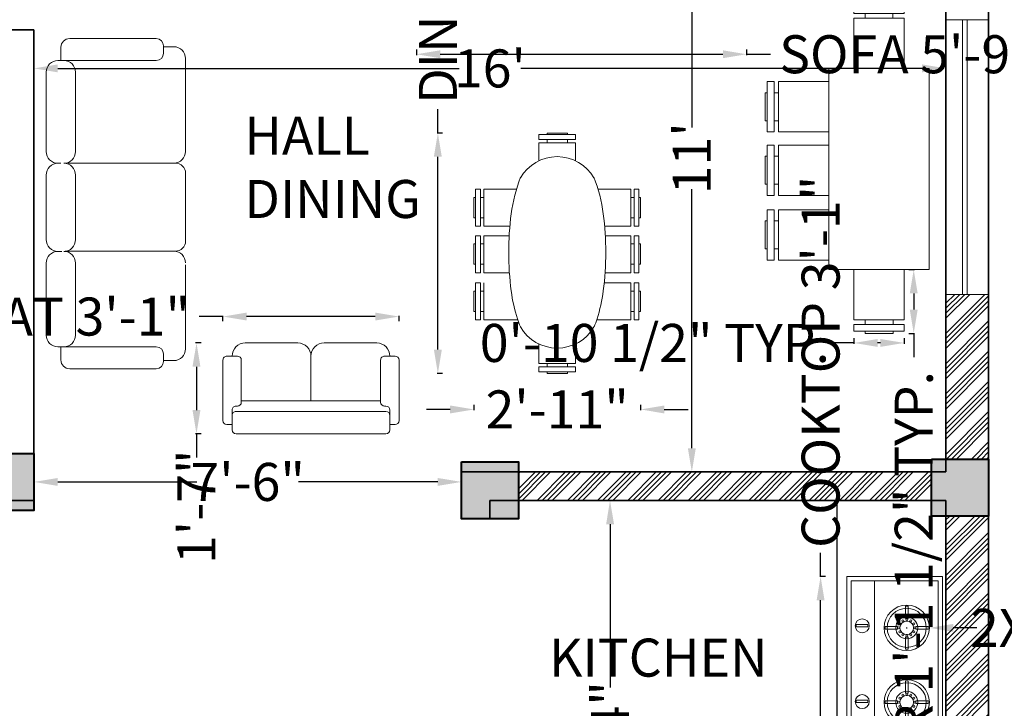
# Model space of a CAD drawing. Units: inches. Extents: x -52 to 493, y -432 to 100.
# Tile 3 of 5: x 163 to 370, y -300 to -155. Entities that reach past the tile are written whole.
import ezdxf

# ---------------------------------------------------------------- set-up
doc = ezdxf.new("R2010")
doc.units = ezdxf.units.IN
doc.header["$MEASUREMENT"] = 0
for name, color, linetype, lineweight in [('A-ANNO-DIMS', 2, 'Continuous', 18), ('A-AREA-IDEN', 7, 'Continuous', 25), ('A-COLS', 7, 'Continuous', 40), ('A-EQPM', 8, 'Continuous', 18), ('A-FLOR-CASE', 8, 'Continuous', 25), ('A-FURN', 8, 'Continuous', 18), ('A-GLAZ', 4, 'Continuous', 18), ('A-WALL', 7, 'Continuous', 35), ('A-WALL-PATT', 8, 'Continuous', 13)]:
    doc.layers.add(name, color=color, linetype=linetype, lineweight=lineweight)
doc.styles.get("Standard").update_dxf_attribs({"font": 'arial.ttf'})
doc.dimstyles.get("Standard").update_dxf_attribs({"dimtxt": 8, "dimasz": 5, "dimexe": 0.18, "dimexo": 0.0625, "dimgap": 0.09, "dimtad": 0, "dimdec": 0, "dimzin": 0, "dimdsep": 46, "dimlunit": 3, "dimtxsty": 'Standard', "dimcen": 0.09, "dimadec": 0, "dimazin": 0, "dimtfac": 1, "dimtdec": 0, "dimtofl": 0, "dimtmove": 0, "dimatfit": 3, "dimfxl": 1, "dimfxlon": 1, "dimtolj": 1, "dimtzin": 0, "dimarcsym": 0})

# ---------------------------------------------------------------- blocks, each defined once
blk = doc.blocks.new('A$C39D66038')
for p, q in [((0.656, 2.02), (0.656, 1.96)), ((1.106, 2.02), (0.656, 2.02)), ((1.106, 1.96), (0.656, 1.96)), ((1.006, 2.04), (0.756, 2.04)), ((0.756, 2.04), (0.756, 2.02)), ((0.756, 1.96), (0.756, 1.92)), ((1.006, 2.02), (1.006, 2.04)), ((1.006, 1.92), (1.006, 1.96)), ((1.106, 1.96), (1.106, 2.02)), ((1.684, 2.02), (1.232, 2.02)), ((1.232, 2.02), (1.232, 1.96)), ((1.684, 1.96), (1.232, 1.96)), ((1.584, 2.04), (1.334, 2.04)), ((1.334, 2.04), (1.334, 2.02)), ((1.334, 1.96), (1.334, 1.92)), ((1.584, 2.02), (1.584, 2.04)), ((1.584, 1.92), (1.584, 1.96)), ((1.684, 1.96), (1.684, 2.02)), ((2.252, 2.02), (1.802, 2.02)), ((1.802, 2.02), (1.802, 1.96)), ((2.252, 1.96), (1.802, 1.96)), ((2.152, 2.04), (1.902, 2.04)), ((1.902, 2.04), (1.902, 2.02)), ((1.902, 1.96), (1.902, 1.92)), ((2.152, 2.02), (2.152, 2.04)), ((2.152, 1.92), (2.152, 1.96)), ((2.252, 1.96), (2.252, 2.02)), ((0.656, 1.92), (0.656, 1.503)), ((1.106, 1.92), (0.656, 1.92)), ((1.232, 1.92), (1.232, 1.606)), ((1.684, 1.92), (1.232, 1.92)), ((1.684, 1.609), (1.684, 1.92)), ((2.252, 1.92), (1.802, 1.92)), ((1.802, 1.92), (1.802, 1.6)), ((2.252, 1.52), (2.252, 1.92)), ((0.02, 1.245), (0.02, 0.795)), ((0.08, 1.245), (0.02, 1.245)), ((0.08, 1.245), (0.08, 0.795)), ((0.12, 1.245), (0.12, 0.795)), ((0.36, 1.245), (0.12, 1.245)), ((2.82, 1.245), (2.6, 1.245)), ((2.82, 0.795), (2.82, 1.245)), ((2.86, 0.795), (2.86, 1.245)), ((2.92, 1.245), (2.86, 1.245)), ((2.92, 0.795), (2.92, 1.245)), ((0, 1.145), (0, 0.895)), ((0.02, 1.145), (0, 1.145)), ((0.12, 1.145), (0.08, 1.145)), ((2.86, 1.145), (2.82, 1.145)), ((2.94, 1.145), (2.92, 1.145)), ((2.94, 0.895), (2.94, 1.145)), ((0, 0.895), (0.02, 0.895)), ((0.08, 0.895), (0.12, 0.895)), ((2.82, 0.895), (2.86, 0.895)), ((2.92, 0.895), (2.94, 0.895)), ((0.02, 0.795), (0.08, 0.795)), ((0.12, 0.795), (0.36, 0.795)), ((2.6, 0.795), (2.82, 0.795)), ((2.86, 0.795), (2.92, 0.795)), ((0.656, 0.537), (0.656, 0.12)), ((2.252, 0.12), (2.252, 0.52)), ((1.106, 0.12), (1.106, 0.445)), ((1.232, 0.434), (1.232, 0.12)), ((1.684, 0.12), (1.684, 0.431)), ((1.802, 0.44), (1.802, 0.12)), ((0.656, 0.12), (1.106, 0.12)), ((0.656, 0.08), (1.106, 0.08)), ((0.656, 0.08), (0.656, 0.02)), ((0.656, 0.02), (1.106, 0.02)), ((0.756, 0.12), (0.756, 0.08)), ((0.756, 0.02), (0.756, 0)), ((1.006, 0.08), (1.006, 0.12)), ((1.006, 0), (1.006, 0.02)), ((1.106, 0.02), (1.106, 0.08)), ((1.232, 0.12), (1.684, 0.12)), ((1.232, 0.08), (1.684, 0.08)), ((1.232, 0.08), (1.232, 0.02)), ((1.232, 0.02), (1.684, 0.02)), ((1.334, 0.12), (1.334, 0.08)), ((1.334, 0.02), (1.334, 0)), ((1.584, 0.08), (1.584, 0.12)), ((1.584, 0), (1.584, 0.02)), ((1.684, 0.02), (1.684, 0.08)), ((1.802, 0.12), (2.252, 0.12)), ((1.802, 0.08), (2.252, 0.08)), ((1.802, 0.08), (1.802, 0.02)), ((1.802, 0.02), (2.252, 0.02)), ((1.902, 0.12), (1.902, 0.08)), ((1.902, 0.02), (1.902, 0)), ((2.152, 0.08), (2.152, 0.12)), ((2.152, 0), (2.152, 0.02)), ((2.252, 0.02), (2.252, 0.08)), ((0.756, 0), (1.006, 0)), ((1.334, 0), (1.584, 0)), ((1.902, 0), (2.152, 0))]:
    blk.add_line(p, q)
for centre, radius, start, end in [((1.267, -0.378), 1.978, 97.5169, 107.6698), ((1.48, -1.99), 3.604, 90, 97.5169), ((1.48, -1.99), 3.604, 82.4831, 90), ((1.693, -0.378), 1.978, 69.0857, 82.4831), ((0.827, 1.02), 0.518, 119.7736, 240.2264), ((0.946, 0.63), 0.921, 107.6698, 114.1273), ((2.133, 1.02), 0.518, 299.7736, 60.2264), ((0.946, 1.41), 0.921, 245.8727, 252.3302), ((1.267, 2.418), 1.978, 252.3302, 262.4831), ((1.693, 2.418), 1.978, 277.5169, 290.9143), ((1.48, 4.03), 3.604, 262.4831, 270), ((1.48, 4.03), 3.604, 270, 277.5169)]:
    blk.add_arc(centre, radius, start, end)
blk = doc.blocks.new('A$C0876780F')
for p, q in [((0.72, 0.95), (0.23, 0.95)), ((1.32, 0.95), (0.88, 0.95)), ((1.48, 0.95), (2.02, 0.95)), ((0.15, 0.85), (0.06, 0.85)), ((0.15, 0.87), (0.15, 0.8444)), ((0.15, 0.87), (0.15, 0.85)), ((0.15, 0.21), (0.15, 0.85)), ((0.8, 0.85), (0.8, 0.87)), ((0.8, 0.87), (0.8, 0.85)), ((0.8, 0.87), (0.8, 0.8444)), ((0.8011, 0.8204), (0.8011, 0.08)), ((1.4, 0.85), (1.4, 0.87)), ((1.4, 0.85), (1.4, 0.87)), ((2.1, 0.87), (2.1, 0.85)), ((2.1, 0.87), (2.1, 0.8444)), ((2.1, 0.21), (2.1, 0.85)), ((2.1, 0.85), (2.19, 0.85)), ((0, 0.79), (0, 0.21)), ((0.72, 0.75), (0.23, 0.75)), ((1.32, 0.75), (0.88, 0.75)), ((1.4014, 0.08), (1.4014, 0.803)), ((1.48, 0.75), (2.02, 0.75)), ((2.25, 0.79), (2.25, 0.21)), ((0, 0.21), (0, 0.2)), ((0.15, 0.2), (0.15, 0.25)), ((2.1, 0.2), (2.1, 0.25)), ((2.25, 0.21), (2.25, 0.2)), ((0.05, 0.15), (0.1, 0.15)), ((0.056, 0.15), (0.056, 0.08)), ((2.2, 0.15), (2.15, 0.15)), ((2.194, 0.15), (2.194, 0.08)), ((0.8011, 0.07), (0.8011, 0.08)), ((1.4014, 0.07), (1.4014, 0.08)), ((0.136, 0), (0.7093, 0)), ((0.8711, 0), (1.3314, 0)), ((2.114, 0), (1.48, 0))]:
    blk.add_line(p, q)
for centre, radius, start, end in [((0.23, 0.87), 0.08, 90, 180), ((0.72, 0.87), 0.08, 0, 90), ((0.88, 0.87), 0.08, 90, 180), ((1.32, 0.87), 0.08, 0, 90), ((1.48, 0.87), 0.08, 90, 180), ((2.02, 0.87), 0.08, 0, 90), ((0.06, 0.79), 0.06, 90, 180), ((0.23, 0.83), 0.08, 180, 270), ((0.23, 0.83), 0.08, 180, 270), ((0.72, 0.83), 0.08, 270, 0), ((0.88, 0.83), 0.08, 180, 270), ((0.88, 0.83), 0.08, 180, 270), ((1.32, 0.83), 0.08, 270, 0), ((1.48, 0.83), 0.08, 180, 270), ((2.02, 0.83), 0.08, 270, 0), ((2.02, 0.83), 0.08, 270, 0), ((2.19, 0.79), 0.06, 0, 90), ((0.09, 0.21), 0.06, 350.53768, 0), ((2.16, 0.21), 0.06, 180, 189.46232), ((0.05, 0.2), 0.05, 180, 270), ((0.1, 0.2), 0.05, 270, 0), ((2.15, 0.2), 0.05, 180, 270), ((2.2, 0.2), 0.05, 270, 0), ((0.136, 0.08), 0.08, 180, 270), ((0.7211, 0.08), 0.08, 270, 0), ((0.8711, 0.07), 0.07, 180, 270), ((1.3314, 0.07), 0.07, 270, 0), ((1.4814, 0.08), 0.08, 180, 270), ((2.114, 0.08), 0.08, 270, 0)]:
    blk.add_arc(centre, radius, start, end)
blk = doc.blocks.new('A$C02A636C4')
for p, q in [((1.2026, 0.6692), (0.097, 0.6692)), ((0.0679, 0.6013), (0.0291, 0.6013)), ((0.0679, 0.6401), (0.0679, 0.6013)), ((0.0679, 0.5334), (0.0679, 0.6013)), ((1.2317, 0.6401), (1.2317, 0.6013)), ((1.2317, 0.6013), (1.2705, 0.6013)), ((1.2317, 0.5334), (1.2317, 0.6013)), ((0, 0.5722), (0, 0.1261)), ((0.0679, 0.4946), (0.0679, 0.5431)), ((1.2317, 0.4946), (1.2317, 0.5431)), ((1.2996, 0.5722), (1.2996, 0.1261)), ((1.2026, 0.5043), (0.097, 0.5043)), ((0.1067, 0.4655), (0.097, 0.4655)), ((0.1358, 0.1261), (0.1358, 0.4364)), ((1.1638, 0.1261), (1.1638, 0.4364)), ((1.1929, 0.4655), (1.2026, 0.4655)), ((1.1638, 0.4267), (0.1358, 0.4267)), ((0.6498, 0.097), (0.6498, 0.4267)), ((0.0291, 0.097), (0.1067, 0.097)), ((1.2705, 0.097), (1.1929, 0.097)), ((0.1649, 0), (0.5528, 0)), ((0.7468, 0), (1.1347, 0))]:
    blk.add_line(p, q)
for centre, radius, start, end in [((0.097, 0.6401), 0.0291, 90, 180), ((1.2026, 0.6401), 0.0291, 0, 90), ((0.0291, 0.5722), 0.0291, 90, 180), ((1.2705, 0.5722), 0.0291, 0, 90), ((0.097, 0.5334), 0.0291, 180, 270), ((1.2026, 0.5334), 0.0291, 270, 0), ((0.097, 0.4946), 0.0291, 180, 270), ((0.1067, 0.4364), 0.0291, 0, 90), ((1.1929, 0.4364), 0.0291, 90, 180), ((1.2026, 0.4946), 0.0291, 270, 0), ((0.0291, 0.1261), 0.0291, 180, 270), ((0.1649, 0.097), 0.097, 180, 270), ((0.1067, 0.1261), 0.0291, 270, 0), ((0.5528, 0.097), 0.097, 270, 0), ((0.7468, 0.097), 0.097, 180, 270), ((1.1347, 0.097), 0.097, 270, 0), ((1.1929, 0.1261), 0.0291, 180, 270), ((1.2705, 0.1261), 0.0291, 270, 0)]:
    blk.add_arc(centre, radius, start, end)
blk = doc.blocks.new('A$C06E242FC')
for p, q in [((0, 455.6), (0.5, 456.1)), ((0, 455.6), (0, 0.5)), ((838.9, 456.1), (0.5, 456.1)), ((20, 435.6), (20.5, 436.1)), ((20, 435.6), (20, 20.5)), ((818.9, 436.1), (20.5, 436.1)), ((819.4, 435.6), (818.9, 436.1)), ((819.4, 20.5), (819.4, 435.6)), ((838.9, 456.1), (839.4, 455.6)), ((839.4, 0.5), (839.4, 455.6)), ((237.3, 411.5), (237.3, 356.2)), ((248.9, 411.5), (237.3, 411.5)), ((248.9, 356.2), (248.9, 411.5)), ((599.3, 411.5), (610.9, 411.5)), ((599.3, 411.5), (599.3, 356.2)), ((610.9, 356.2), (610.9, 411.5)), ((237.3, 356.2), (248.9, 356.2)), ((599.3, 356.2), (610.9, 356.2)), ((20, 324.4), (819.4, 324.4)), ((232.7, 272.7), (232.7, 214)), ((244.9, 272.7), (232.7, 272.7)), ((244.9, 214), (244.9, 272.7)), ((588.1, 272.7), (588.1, 214)), ((600.3, 272.7), (588.1, 272.7)), ((600.3, 214), (600.3, 272.7)), ((232.7, 214), (244.9, 214)), ((588.1, 214), (600.3, 214)), ((136.3, 176), (136.3, 163.8)), ((194.9, 176), (136.3, 176)), ((136.3, 163.8), (194.9, 163.8)), ((194.9, 163.8), (194.9, 176)), ((282.9, 176.3), (282.9, 164.1)), ((341.6, 176.3), (282.9, 176.3)), ((282.9, 164.1), (341.6, 164.1)), ((341.6, 164.1), (341.6, 176.3)), ((550.3, 176), (491.7, 176)), ((491.7, 176), (491.7, 163.8)), ((491.7, 163.8), (550.3, 163.8)), ((550.3, 163.8), (550.3, 176)), ((638.3, 176.3), (638.3, 164.1)), ((697, 176.3), (638.3, 176.3)), ((638.3, 164.1), (697, 164.1)), ((697, 164.1), (697, 176.3)), ((245.2, 126.1), (233, 126.1)), ((233, 126.1), (233, 67.4)), ((245.2, 67.4), (245.2, 126.1)), ((600.6, 126.1), (588.3, 126.1)), ((588.3, 126.1), (588.3, 67.4)), ((600.6, 67.4), (600.6, 126.1)), ((233, 67.4), (245.2, 67.4)), ((588.3, 67.4), (600.6, 67.4)), ((0, 0.5), (0.5, 0)), ((20, 20.5), (20.5, 20)), ((20.5, 20), (818.9, 20)), ((818.9, 20), (819.4, 20.5)), ((838.9, 0), (839.4, 0.5)), ((0.5, 0), (838.9, 0))]:
    blk.add_line(p, q)
for centre, radius in [((242, 382.9), 33.3), ((604.1, 382.9), 33.3), ((238.9, 170.1), 108.3), ((238.9, 170.1), 93.3), ((594.3, 170.1), 108.3), ((594.3, 170.1), 93.3), ((238.9, 170.1), 52.6), ((205.3, 189.5), 4.84), ((238.9, 170.1), 32.6), ((219.5, 203.7), 4.84), ((238.9, 208.9), 4.84), ((258.4, 203.7), 4.84), ((272.6, 189.5), 4.84), ((594.3, 170.1), 52.6), ((560.7, 189.5), 4.84), ((594.3, 170.1), 32.6), ((574.9, 203.7), 4.84), ((594.3, 208.9), 4.84), ((613.7, 203.7), 4.84), ((628, 189.5), 4.84), ((200.1, 170.1), 4.84), ((205.3, 150.6), 4.84), ((219.5, 136.4), 4.84), ((258.4, 136.4), 4.84), ((272.6, 150.6), 4.84), ((277.8, 170.1), 4.84), ((555.5, 170.1), 4.84), ((560.7, 150.6), 4.84), ((574.9, 136.4), 4.84), ((613.7, 136.4), 4.84), ((628, 150.6), 4.84), ((633.2, 170.1), 4.84), ((238.9, 131.2), 4.84), ((594.3, 131.2), 4.84)]:
    blk.add_circle(centre, radius)
blk = doc.blocks.new('*D19')
at = {"layer": 'A-ANNO-DIMS', "color": 0, "lineweight": -2, "transparency": 16777216}
for p, q in [((285.94, -256.62), (287.12, -256.62)), ((286.94, -261.62), (286.94, -295.94)), ((286.94, -351.72), (286.94, -317.4)), ((285.94, -356.72), (287.12, -356.72))]:
    blk.add_line(p, q, dxfattribs=at)
at = {"layer": 'A-ANNO-DIMS', "color": 0, "transparency": 16777216}
for points in [[(286.11, -261.62), (287.78, -261.62), (286.94, -256.62)], [(286.11, -351.72), (287.78, -351.72), (286.94, -356.72)]]:
    blk.add_solid(points, dxfattribs=at)
at = {"layer": 'Defpoints', "color": 0, "transparency": 16777216}
for p in [(283.02, -256.62), (280.41, -356.72), (286.94, -356.72)]:
    blk.add_point(p, dxfattribs=at)
at = {"layer": 'A-ANNO-DIMS', "color": 0, "transparency": 16777216, "insert": (286.94, -306.67), "char_height": 8, "attachment_point": 5, "rotation": 90}
blk.add_mtext('\\A1;8\'-4"', dxfattribs=at)
blk = doc.blocks.new('*D24')
at = {"layer": 'A-ANNO-DIMS', "color": 0, "lineweight": -2, "transparency": 16777216}
for p, q in [((165.65, -252.71), (165.65, -252.53)), ((170.65, -252.71), (199.96, -252.71)), ((250.65, -252.71), (221.34, -252.71)), ((255.65, -252.71), (255.65, -252.53))]:
    blk.add_line(p, q, dxfattribs=at)
at = {"layer": 'A-ANNO-DIMS', "color": 0, "transparency": 16777216}
for points in [[(170.65, -251.88), (170.65, -253.54), (165.65, -252.71)], [(250.65, -251.88), (250.65, -253.54), (255.65, -252.71)]]:
    blk.add_solid(points, dxfattribs=at)
at = {"layer": 'Defpoints', "color": 0, "transparency": 16777216}
for p in [(165.65, -252.71), (255.65, -252.71), (255.65, -252.71)]:
    blk.add_point(p, dxfattribs=at)
at = {"layer": 'A-ANNO-DIMS', "color": 0, "transparency": 16777216, "insert": (210.65, -252.71), "char_height": 8, "attachment_point": 5}
blk.add_mtext('\\A1;7\'-6"', dxfattribs=at)
blk = doc.blocks.new('*D25')
at = {"layer": 'A-ANNO-DIMS', "color": 0, "lineweight": -2, "transparency": 16777216}
for p, q in [((165.65, -164.71), (165.65, -165.89)), ((170.65, -165.71), (255.15, -165.71)), ((352.65, -165.71), (268.15, -165.71)), ((357.65, -164.71), (357.65, -165.89))]:
    blk.add_line(p, q, dxfattribs=at)
at = {"layer": 'A-ANNO-DIMS', "color": 0, "transparency": 16777216}
for points in [[(170.65, -164.87), (170.65, -166.54), (165.65, -165.71)], [(352.65, -164.87), (352.65, -166.54), (357.65, -165.71)]]:
    blk.add_solid(points, dxfattribs=at)
at = {"layer": 'Defpoints', "color": 0, "transparency": 16777216}
for p in [(357.65, -155.46), (165.65, -160.73), (357.65, -165.71)]:
    blk.add_point(p, dxfattribs=at)
at = {"layer": 'A-ANNO-DIMS', "color": 0, "transparency": 16777216, "insert": (261.65, -165.71), "char_height": 8, "attachment_point": 5}
blk.add_mtext("\\A1;16'", dxfattribs=at)
blk = doc.blocks.new('*D26')
at = {"layer": 'A-ANNO-DIMS', "color": 0, "lineweight": -2, "transparency": 16777216}
for p, q in [((305.16, -118.62), (303.98, -118.62)), ((304.16, -123.62), (304.16, -178.11)), ((304.16, -245.62), (304.16, -191.12)), ((305.16, -250.62), (303.98, -250.62))]:
    blk.add_line(p, q, dxfattribs=at)
at = {"layer": 'A-ANNO-DIMS', "color": 0, "transparency": 16777216}
for points in [[(303.33, -123.62), (305, -123.62), (304.16, -118.62)], [(303.33, -245.62), (305, -245.62), (304.16, -250.62)]]:
    blk.add_solid(points, dxfattribs=at)
at = {"layer": 'Defpoints', "color": 0, "transparency": 16777216}
for p in [(304.16, -118.62), (307.2, -118.62), (312.14, -250.62)]:
    blk.add_point(p, dxfattribs=at)
at = {"layer": 'A-ANNO-DIMS', "color": 0, "transparency": 16777216, "insert": (304.16, -184.62), "char_height": 8, "attachment_point": 5, "rotation": 90}
blk.add_mtext("\\A1;11'", dxfattribs=at)
blk = doc.blocks.new('COL-12X12')
h = blk.add_hatch(color=256)
h.dxf.hatch_style = 1
h.paths.add_polyline_path([(12, 12), (0, 12), (0, 0), (12, 0)])
blk.add_lwpolyline([(0, 12), (12, 12), (12, 0), (0, 0)], close=True)
blk = doc.blocks.new('WIN-SIDE-58')
for p, q in [((0, 57.79), (9, 57.79)), ((3.5, 0), (3.5, 57.79)), ((4.5, 0), (4.5, 57.79)), ((0, 0), (9, 0))]:
    blk.add_line(p, q)
blk = doc.blocks.new('CHAIR-DINING')
for p, q in [((10.59, 12.94), (0, 12.94)), ((0, 12.94), (0, 11.53)), ((8.23, 13.41), (2.35, 13.41)), ((2.35, 13.41), (2.35, 12.94)), ((8.23, 12.94), (8.23, 13.41)), ((10.59, 11.53), (10.59, 12.94)), ((10.59, 11.53), (0, 11.53)), ((10.59, 10.59), (0, 10.59)), ((0, 10.59), (0, 0)), ((2.35, 11.53), (2.35, 10.59)), ((8.23, 10.59), (8.23, 11.53)), ((10.59, 0), (10.59, 10.59)), ((0, 0), (10.59, 0))]:
    blk.add_line(p, q)
blk = doc.blocks.new('*D44')
at = {"layer": 'A-ANNO-DIMS', "color": 0, "lineweight": -2, "transparency": 16777216}
for p, q in [((349.88, -208.05), (351.06, -208.05)), ((350.88, -213.05), (350.88, -216.46)), ((349.88, -221.46), (351.06, -221.46)), ((350.88, -221.46), (350.88, -226.46))]:
    blk.add_line(p, q, dxfattribs=at)
at = {"layer": 'A-ANNO-DIMS', "color": 0, "transparency": 16777216}
for points in [[(350.04, -213.05), (351.71, -213.05), (350.88, -208.05)], [(350.04, -216.46), (351.71, -216.46), (350.88, -221.46)]]:
    blk.add_solid(points, dxfattribs=at)
at = {"layer": 'Defpoints', "color": 0, "transparency": 16777216}
for p in [(348.87, -208.05), (348.87, -221.46), (350.88, -221.46)]:
    blk.add_point(p, dxfattribs=at)
at = {"layer": 'A-ANNO-DIMS', "color": 0, "transparency": 16777216, "insert": (350.88, -300.1), "char_height": 8, "attachment_point": 5, "rotation": 90}
blk.add_mtext('\\A1;DINING CHAIR 1\'-1 1/2" TYP.', dxfattribs=at)
blk = doc.blocks.new('*D45')
at = {"layer": 'A-ANNO-DIMS', "color": 0, "lineweight": -2, "transparency": 16777216}
for p, q in [((338.28, -223.47), (333.28, -223.47)), ((338.28, -222.47), (338.28, -223.65)), ((343.87, -223.47), (343.28, -223.47)), ((348.87, -222.47), (348.87, -223.65))]:
    blk.add_line(p, q, dxfattribs=at)
at = {"layer": 'A-ANNO-DIMS', "color": 0, "transparency": 16777216}
for points in [[(343.28, -222.64), (343.28, -224.3), (338.28, -223.47)], [(343.87, -222.64), (343.87, -224.3), (348.87, -223.47)]]:
    blk.add_solid(points, dxfattribs=at)
at = {"layer": 'Defpoints', "color": 0, "transparency": 16777216}
for p in [(338.28, -221.46), (348.87, -221.46), (338.28, -223.47)]:
    blk.add_point(p, dxfattribs=at)
at = {"layer": 'A-ANNO-DIMS', "color": 0, "transparency": 16777216, "insert": (296.38, -223.47), "char_height": 8, "attachment_point": 5}
blk.add_mtext('\\A1;0\'-10 1/2" TYP.', dxfattribs=at)
blk = doc.blocks.new('*D46')
at = {"layer": 'A-ANNO-DIMS', "color": 0, "lineweight": -2, "transparency": 16777216}
for p, q in [((246.2, -161.73), (246.2, -162.91)), ((251.2, -162.73), (310.69, -162.73)), ((315.69, -161.73), (315.69, -162.91)), ((315.69, -162.73), (320.69, -162.73))]:
    blk.add_line(p, q, dxfattribs=at)
at = {"layer": 'A-ANNO-DIMS', "color": 0, "transparency": 16777216}
for points in [[(251.2, -161.9), (251.2, -163.56), (246.2, -162.73)], [(310.69, -161.9), (310.69, -163.56), (315.69, -162.73)]]:
    blk.add_solid(points, dxfattribs=at)
at = {"layer": 'Defpoints', "color": 0, "transparency": 16777216}
for p in [(246.2, -152.31), (315.69, -152.31), (315.69, -162.73)]:
    blk.add_point(p, dxfattribs=at)
at = {"layer": 'A-ANNO-DIMS', "color": 0, "transparency": 16777216, "insert": (371.23, -162.73), "char_height": 8, "attachment_point": 5}
blk.add_mtext('\\A1;SOFA 5\'-9 1/2" TYP.', dxfattribs=at)
blk = doc.blocks.new('*D48')
at = {"layer": 'A-ANNO-DIMS', "color": 0, "lineweight": -2, "transparency": 16777216}
for p, q in [((250.69, -179.3), (250.69, -174.3)), ((251.69, -179.3), (250.51, -179.3)), ((250.69, -224.88), (250.69, -184.3)), ((251.69, -229.88), (250.51, -229.88))]:
    blk.add_line(p, q, dxfattribs=at)
at = {"layer": 'A-ANNO-DIMS', "color": 0, "transparency": 16777216}
for points in [[(249.85, -184.3), (251.52, -184.3), (250.69, -179.3)], [(249.85, -224.88), (251.52, -224.88), (250.69, -229.88)]]:
    blk.add_solid(points, dxfattribs=at)
at = {"layer": 'Defpoints', "color": 0, "transparency": 16777216}
for p in [(250.69, -179.3), (258.27, -179.3), (258.27, -229.88)]:
    blk.add_point(p, dxfattribs=at)
at = {"layer": 'A-ANNO-DIMS', "color": 0, "transparency": 16777216, "insert": (250.69, -120.92), "char_height": 8, "attachment_point": 5, "rotation": 90}
blk.add_mtext('\\A1;DINING SET 4\'-2 1/2"', dxfattribs=at)
blk = doc.blocks.new('*D49')
at = {"layer": 'A-ANNO-DIMS', "color": 0, "lineweight": -2, "transparency": 16777216}
for p, q in [((253.27, -237.46), (248.27, -237.46)), ((258.27, -236.46), (258.27, -237.64)), ((293.37, -236.46), (293.37, -237.64)), ((298.37, -237.46), (303.37, -237.46))]:
    blk.add_line(p, q, dxfattribs=at)
at = {"layer": 'A-ANNO-DIMS', "color": 0, "transparency": 16777216}
for points in [[(253.27, -236.63), (253.27, -238.3), (258.27, -237.46)], [(298.37, -236.63), (298.37, -238.3), (293.37, -237.46)]]:
    blk.add_solid(points, dxfattribs=at)
at = {"layer": 'Defpoints', "color": 0, "transparency": 16777216}
for p in [(258.27, -229.88), (293.37, -229.88), (258.27, -237.46)]:
    blk.add_point(p, dxfattribs=at)
at = {"layer": 'A-ANNO-DIMS', "color": 0, "transparency": 16777216, "insert": (275.82, -237.46), "char_height": 8, "attachment_point": 5}
blk.add_mtext('\\A1;2\'-11"', dxfattribs=at)
blk = doc.blocks.new('*D50')
at = {"layer": 'A-ANNO-DIMS', "color": 0, "lineweight": -2, "transparency": 16777216}
for p, q in [((205.43, -217.92), (200.43, -217.92)), ((205.43, -218.92), (205.43, -217.74)), ((237.52, -217.92), (210.43, -217.92)), ((242.52, -218.92), (242.52, -217.74))]:
    blk.add_line(p, q, dxfattribs=at)
at = {"layer": 'A-ANNO-DIMS', "color": 0, "transparency": 16777216}
for points in [[(210.43, -217.09), (210.43, -218.75), (205.43, -217.92)], [(237.52, -217.09), (237.52, -218.75), (242.52, -217.92)]]:
    blk.add_solid(points, dxfattribs=at)
at = {"layer": 'Defpoints', "color": 0, "transparency": 16777216}
for p in [(205.43, -217.92), (205.43, -223.48), (242.52, -223.48)]:
    blk.add_point(p, dxfattribs=at)
at = {"layer": 'A-ANNO-DIMS', "color": 0, "transparency": 16777216, "insert": (158.83, -217.92), "char_height": 8, "attachment_point": 5}
blk.add_mtext('\\A1;LOVESEAT 3\'-1"', dxfattribs=at)
blk = doc.blocks.new('*D51')
at = {"layer": 'A-ANNO-DIMS', "color": 0, "lineweight": -2, "transparency": 16777216}
for p, q in [((200.87, -223.48), (199.69, -223.48)), ((199.87, -228.48), (199.87, -237.58)), ((200.87, -242.58), (199.69, -242.58)), ((199.87, -242.58), (199.87, -247.58))]:
    blk.add_line(p, q, dxfattribs=at)
at = {"layer": 'A-ANNO-DIMS', "color": 0, "transparency": 16777216}
for points in [[(199.03, -228.48), (200.7, -228.48), (199.87, -223.48)], [(199.03, -237.58), (200.7, -237.58), (199.87, -242.58)]]:
    blk.add_solid(points, dxfattribs=at)
at = {"layer": 'Defpoints', "color": 0, "transparency": 16777216}
for p in [(205.43, -223.48), (199.87, -242.58), (205.43, -242.58)]:
    blk.add_point(p, dxfattribs=at)
at = {"layer": 'A-ANNO-DIMS', "color": 0, "transparency": 16777216, "insert": (199.87, -257.93), "char_height": 8, "attachment_point": 5, "rotation": 90}
blk.add_mtext('\\A1;1\'-7"', dxfattribs=at)
blk = doc.blocks.new('*D54')
at = {"layer": 'A-ANNO-DIMS', "color": 0, "lineweight": -2, "transparency": 16777216}
for p, q in [((331.27, -272.61), (331.27, -267.61)), ((332.27, -272.61), (331.09, -272.61)), ((331.27, -304.59), (331.27, -277.61)), ((332.27, -309.59), (331.09, -309.59))]:
    blk.add_line(p, q, dxfattribs=at)
at = {"layer": 'A-ANNO-DIMS', "color": 0, "transparency": 16777216}
for points in [[(330.43, -277.61), (332.1, -277.61), (331.27, -272.61)], [(330.43, -304.59), (332.1, -304.59), (331.27, -309.59)]]:
    blk.add_solid(points, dxfattribs=at)
at = {"layer": 'Defpoints', "color": 0, "transparency": 16777216}
for p in [(331.27, -272.61), (336.81, -272.61), (336.81, -309.59)]:
    blk.add_point(p, dxfattribs=at)
at = {"layer": 'A-ANNO-DIMS', "color": 0, "transparency": 16777216, "insert": (331.27, -227.44), "char_height": 8, "attachment_point": 5, "rotation": 90}
blk.add_mtext('\\A1;COOKTOP 3\'-1"', dxfattribs=at)
blk = doc.blocks.new('*D62')
at = {"layer": 'A-ANNO-DIMS', "color": 0, "lineweight": -2, "transparency": 16777216}
for p, q in [((390.3, -213.25), (390.3, -208.25)), ((389.3, -213.25), (390.48, -213.25)), ((390.3, -242.89), (390.3, -218.25)), ((389.3, -247.89), (390.48, -247.89))]:
    blk.add_line(p, q, dxfattribs=at)
at = {"layer": 'A-ANNO-DIMS', "color": 0, "transparency": 16777216}
for points in [[(389.46, -218.25), (391.13, -218.25), (390.3, -213.25)], [(389.46, -242.89), (391.13, -242.89), (390.3, -247.89)]]:
    blk.add_solid(points, dxfattribs=at)
at = {"layer": 'Defpoints', "color": 0, "transparency": 16777216}
for p in [(366.65, -213.25), (390.3, -213.25), (366.65, -247.89)]:
    blk.add_point(p, dxfattribs=at)
at = {"layer": 'A-ANNO-DIMS', "color": 0, "transparency": 16777216, "insert": (390.3, -185.03), "char_height": 8, "attachment_point": 5, "rotation": 90}
blk.add_mtext('\\A1;2\'-10 1/2"', dxfattribs=at)
blk = doc.blocks.new('*D73')
at = {"layer": 'A-ANNO-DIMS', "color": 0, "lineweight": -2, "transparency": 16777216}
for p, q in [((389.3, -260.49), (390.48, -260.49)), ((390.3, -265.49), (390.3, -269.69)), ((390.3, -295.34), (390.3, -291.13)), ((389.3, -300.34), (390.48, -300.34))]:
    blk.add_line(p, q, dxfattribs=at)
at = {"layer": 'A-ANNO-DIMS', "color": 0, "transparency": 16777216}
for points in [[(389.46, -265.49), (391.13, -265.49), (390.3, -260.49)], [(389.46, -295.34), (391.13, -295.34), (390.3, -300.34)]]:
    blk.add_solid(points, dxfattribs=at)
at = {"layer": 'Defpoints', "color": 0, "transparency": 16777216}
for p in [(261.65, -260.49), (261.65, -300.34), (390.3, -300.34)]:
    blk.add_point(p, dxfattribs=at)
at = {"layer": 'A-ANNO-DIMS', "color": 0, "transparency": 16777216, "insert": (390.3, -280.41), "char_height": 8, "attachment_point": 5, "rotation": 90}
blk.add_mtext('\\A1;3\'-4"', dxfattribs=at)
blk = doc.blocks.new('*D74')
at = {"layer": 'A-ANNO-DIMS', "color": 0, "lineweight": -2, "transparency": 16777216}
for p, q in [((334.72, 87.29), (334.72, 88.47)), ((339.72, 88.29), (352.65, 88.29)), ((357.65, 87.29), (357.65, 88.47)), ((357.65, 88.29), (362.65, 88.29))]:
    blk.add_line(p, q, dxfattribs=at)
at = {"layer": 'A-ANNO-DIMS', "color": 0, "transparency": 16777216}
for points in [[(339.72, 89.13), (339.72, 87.46), (334.72, 88.29)], [(352.65, 89.13), (352.65, 87.46), (357.65, 88.29)]]:
    blk.add_solid(points, dxfattribs=at)
at = {"layer": 'Defpoints', "color": 0, "transparency": 16777216}
for p in [(357.65, 88.29), (334.72, -335.93), (357.65, -358.62)]:
    blk.add_point(p, dxfattribs=at)
at = {"layer": 'A-ANNO-DIMS', "color": 0, "transparency": 16777216, "insert": (376.1, 88.29), "char_height": 8, "attachment_point": 5}
blk.add_mtext('\\A1;1\'-11"', dxfattribs=at)
blk = doc.blocks.new('*D76')
at = {"layer": 'A-ANNO-DIMS', "color": 0, "lineweight": -2, "transparency": 16777216}
for p, q in [((327.99, -420.22), (322.99, -420.22)), ((332.99, -419.22), (332.99, -420.4)), ((354.16, -419.22), (354.16, -420.4)), ((359.16, -420.22), (364.16, -420.22))]:
    blk.add_line(p, q, dxfattribs=at)
at = {"layer": 'A-ANNO-DIMS', "color": 0, "transparency": 16777216}
for points in [[(327.99, -419.39), (327.99, -421.06), (332.99, -420.22)], [(359.16, -419.39), (359.16, -421.06), (354.16, -420.22)]]:
    blk.add_solid(points, dxfattribs=at)
at = {"layer": 'Defpoints', "color": 0, "transparency": 16777216}
for p in [(332.99, -208.05), (354.16, -208.05), (354.16, -420.22)]:
    blk.add_point(p, dxfattribs=at)
at = {"layer": 'A-ANNO-DIMS', "color": 0, "transparency": 16777216, "insert": (343.57, -420.22), "char_height": 8, "attachment_point": 5}
blk.add_mtext('\\A1;1\'-9"', dxfattribs=at)
blk = doc.blocks.new('*D77')
at = {"layer": 'A-ANNO-DIMS', "color": 0, "lineweight": -2, "transparency": 16777216}
for p, q in [((390.3, -160.71), (390.3, -155.71)), ((389.3, -165.71), (390.48, -165.71)), ((389.3, -208.05), (390.48, -208.05)), ((390.3, -213.05), (390.3, -218.05))]:
    blk.add_line(p, q, dxfattribs=at)
at = {"layer": 'A-ANNO-DIMS', "color": 0, "transparency": 16777216}
for points in [[(389.46, -160.71), (391.13, -160.71), (390.3, -165.71)], [(389.46, -213.05), (391.13, -213.05), (390.3, -208.05)]]:
    blk.add_solid(points, dxfattribs=at)
at = {"layer": 'Defpoints', "color": 0, "transparency": 16777216}
for p in [(354.16, -165.71), (354.16, -208.05), (390.3, -208.05)]:
    blk.add_point(p, dxfattribs=at)
at = {"layer": 'A-ANNO-DIMS', "color": 0, "transparency": 16777216, "insert": (390.3, -186.88), "char_height": 8, "attachment_point": 5, "rotation": 90}
blk.add_mtext('\\A1;3\'-6 1/2"', dxfattribs=at)
blk = doc.blocks.new('*D79')
at = {"layer": 'A-ANNO-DIMS', "color": 0, "lineweight": -2, "transparency": 16777216}
for p, q in [((181.73, -419.22), (181.73, -420.4)), ((186.73, -420.22), (192.57, -420.22)), ((197.57, -419.22), (197.57, -420.4)), ((197.57, -420.22), (202.57, -420.22))]:
    blk.add_line(p, q, dxfattribs=at)
at = {"layer": 'A-ANNO-DIMS', "color": 0, "transparency": 16777216}
for points in [[(186.73, -419.39), (186.73, -421.06), (181.73, -420.22)], [(192.57, -419.39), (192.57, -421.06), (197.57, -420.22)]]:
    blk.add_solid(points, dxfattribs=at)
at = {"layer": 'Defpoints', "color": 0, "transparency": 16777216}
for p in [(181.73, 19.38), (197.57, 19.38), (197.57, -420.22)]:
    blk.add_point(p, dxfattribs=at)
at = {"layer": 'A-ANNO-DIMS', "color": 0, "transparency": 16777216, "insert": (212.91, -420.22), "char_height": 8, "attachment_point": 5}
blk.add_mtext('\\A1;1\'-4"', dxfattribs=at)
blk = doc.blocks.new('*D81')
at = {"layer": 'A-ANNO-DIMS', "color": 0, "lineweight": -2, "transparency": 16777216}
for p, q in [((154.65, -420.22), (149.65, -420.22)), ((159.65, -419.22), (159.65, -420.4)), ((165.65, -419.22), (165.65, -420.4)), ((170.65, -420.22), (175.65, -420.22))]:
    blk.add_line(p, q, dxfattribs=at)
at = {"layer": 'A-ANNO-DIMS', "color": 0, "transparency": 16777216}
for points in [[(154.65, -419.39), (154.65, -421.06), (159.65, -420.22)], [(170.65, -419.39), (170.65, -421.06), (165.65, -420.22)]]:
    blk.add_solid(points, dxfattribs=at)
at = {"layer": 'Defpoints', "color": 0, "transparency": 16777216}
for p in [(159.65, -79.87), (165.65, -79.87), (165.65, -420.22)]:
    blk.add_point(p, dxfattribs=at)
at = {"layer": 'A-ANNO-DIMS', "color": 0, "transparency": 16777216, "insert": (186.37, -420.22), "char_height": 8, "attachment_point": 5}
blk.add_mtext('\\A1;0\'-6"', dxfattribs=at)
blk = doc.blocks.new('*D84')
at = {"layer": 'A-ANNO-DIMS', "color": 0, "lineweight": -2, "transparency": 16777216}
for p, q in [((349.33, -283.41), (349.51, -283.41)), ((349.42, -283.5), (349.42, -283.32)), ((364.19, -283.41), (359.19, -283.41))]:
    blk.add_line(p, q, dxfattribs=at)
at = {"layer": 'A-ANNO-DIMS', "color": 0, "transparency": 16777216}
blk.add_solid([(359.19, -282.58), (359.19, -284.25), (354.19, -283.41)], dxfattribs=at)
at = {"layer": 'Defpoints', "color": 0, "transparency": 16777216}
for p in [(344.65, -283.41), (354.19, -283.41)]:
    blk.add_point(p, dxfattribs=at)
at = {"layer": 'A-ANNO-DIMS', "color": 0, "transparency": 16777216, "insert": (397.03, -283.42), "char_height": 8, "attachment_point": 5, "rotation": 359.9944}
blk.add_mtext('\\A1;2X ∅0\'-9 1/2"', dxfattribs=at)

msp = doc.modelspace()

# ---------------------------------------------------------------- hatches: boundary and pattern name
at = {"layer": 'A-WALL-PATT'}
h = msp.add_hatch(dxfattribs=at)
h.set_pattern_fill('ANSI34', color=256, scale=6)
h.paths.add_polyline_path([(366.65, -213.25), (357.65, -213.25), (357.65, -247.89), (366.65, -247.89)])
h.paths.add_polyline_path([(354.65, -250.62), (267.65, -250.62), (267.65, -256.62), (354.65, -256.62)])
h.paths.add_polyline_path([(366.65, -259.89), (357.65, -259.89), (357.65, -352.62), (366.65, -352.62)])
h.paths.add_polyline_path([(354.65, -358.62), (331.2, -358.62), (331.2, -364.62), (354.65, -364.62)])
h.paths.add_polyline_path([(288.89, -358.62), (267.65, -358.62), (267.65, -364.62), (288.89, -364.62)])
h.paths.add_polyline_path([(153.65, -358.62), (101.4, -358.62), (101.4, -364.62), (153.65, -364.62)])
h.paths.add_polyline_path([(59.09, -358.62), (18.65, -358.62), (18.65, -364.62), (59.09, -364.62)])
h.paths.add_polyline_path([(15.65, -259.14), (6.65, -259.14), (6.65, -352.62), (15.65, -352.62)])
h.paths.add_polyline_path([(153.65, -250.62), (18.65, -250.62), (18.65, -256.62), (153.65, -256.62)])
h.paths.add_polyline_path([(15.65, -213.25), (6.65, -213.25), (6.65, -247.14), (15.65, -247.14)])
h.paths.add_polyline_path([(15.65, -121.57), (6.65, -121.57), (6.65, -155.46), (15.65, -155.46), (15.65, -143.44)])

# ---------------------------------------------------------------- linework, layer by layer
at = {"layer": 'A-FLOR-CASE'}
msp.add_line((334.72, -256.62), (334.72, -335.93), dxfattribs=at)
at = {"layer": 'A-FURN'}
for p, q in [((332.99, -165.71), (354.16, -165.71)), ((332.99, -165.71), (332.99, -208.05)), ((354.16, -208.05), (354.16, -165.71)), ((320.05, -181.84), (320.05, -192.47)), ((321.46, -181.84), (320.05, -181.84)), ((321.46, -181.84), (321.46, -192.47)), ((332.99, -181.84), (322.4, -181.84)), ((322.4, -181.84), (322.4, -192.47)), ((332.99, -195.42), (332.99, -181.84)), ((319.58, -184.19), (319.58, -190.07)), ((320.05, -184.19), (319.58, -184.19)), ((322.4, -184.19), (321.46, -184.19)), ((319.58, -190.07), (320.05, -190.07)), ((321.46, -190.07), (322.4, -190.07)), ((320.05, -192.47), (321.46, -192.47)), ((322.4, -192.47), (332.99, -192.47)), ((332.99, -208.05), (354.16, -208.05))]:
    msp.add_line(p, q, dxfattribs=at)
at = {"layer": 'A-WALL'}
for p, q in [((366.65, 28.38), (366.65, -364.62)), ((357.65, 19.38), (357.65, -250.62)), ((165.65, -157.57), (159.65, -157.57)), ((165.65, -157.57), (165.65, -256.62)), ((255.65, -250.62), (357.65, -250.62)), ((255.65, -250.62), (255.65, -260.49)), ((15.65, -256.62), (165.65, -256.62)), ((261.65, -256.62), (357.65, -256.62)), ((261.65, -256.62), (261.65, -260.49)), ((357.65, -256.62), (357.65, -358.62))]:
    msp.add_line(p, q, dxfattribs=at)

# ---------------------------------------------------------------- block references
at = {"layer": 'A-COLS'}
for p in [(153.65, -258.71), (255.65, -260.49), (354.65, -259.89)]:
    msp.add_blockref('COL-12X12', p, dxfattribs=at)
at = {"layer": 'A-EQPM', "xscale": 0.0440556486278997, "yscale": 0.0440556486278997, "zscale": 0.0440556486278997, "rotation": 90}
msp.add_blockref('A$C06E242FC', (356.91, -309.59), dxfattribs=at)
at = {"layer": 'A-FURN'}
msp.add_blockref('CHAIR-DINING', (338.28, -165.71), dxfattribs=at)
for name, p, xscale, yscale, zscale, rotation in [('A$C0876780F', (197.57, -228.91), 30.88339250666864, 30.88339250666864, 30.88339250666864, 90), ('A$C39D66038', (293.37, -229.88), 17.20422601796143, 17.20422601796143, 17.20422601796143, 90), ('A$C02A636C4', (242.52, -223.48), 28.53485635951324, 28.53485635951324, 28.53485635951324, 180)]:
    msp.add_blockref(name, p, dxfattribs=dict(at, xscale=xscale, yscale=yscale, zscale=zscale, rotation=rotation))
for p, rotation in [((332.99, -179.06), 89.99999999992728), ((332.99, -206.03), 90.00000000019013), ((348.87, -208.05), 180)]:
    msp.add_blockref('CHAIR-DINING', p, dxfattribs=dict(at, rotation=rotation))
at = {"layer": 'A-GLAZ'}
msp.add_blockref('WIN-SIDE-58', (357.65, -213.25), dxfattribs=at)

# ---------------------------------------------------------------- texts
at = {"layer": 'A-AREA-IDEN', "char_height": 8, "attachment_point": 1}
for s, insert in [('HALL\\PDINING', (209.93, -175.85)), ('KITCHEN', (274.09, -285.68))]:
    msp.add_mtext_dynamic_manual_height_columns(s, width=75.9525, gutter_width=1, heights=[0], dxfattribs=dict(at, insert=insert))

# ---------------------------------------------------------------- dimensions: what is measured, and where the dimension line sits
at = {"layer": 'A-ANNO-DIMS'}
for base, p1, p2, override, picture, middle in [((357.65, 88.29), (334.72, -335.93), (357.65, -358.62), {"dimdec": 1, "dimlfac": 1, "dimrnd": 0, "dimzin": 1, "dimdsep": 46, "dimlunit": 4, "dimfrac": 2}, '*D74', (376.1, 88.29)), ((197.57, -420.22), (181.73, 19.38), (197.57, 19.38), {"dimdec": 1, "dimlfac": 1, "dimrnd": 0, "dimzin": 1, "dimdsep": 46, "dimlunit": 4, "dimfrac": 2}, '*D79', (212.91, -420.22)), ((165.65, -420.22), (159.65, -79.87), (165.65, -79.87), {"dimdec": 1, "dimlfac": 1, "dimrnd": 0, "dimzin": 1, "dimdsep": 46, "dimlunit": 4, "dimfrac": 2}, '*D81', (186.37, -420.22)), ((357.65, -165.71), (165.65, -160.73), (357.65, -155.46), {"dimclrd": 0, "dimclre": 0, "dimclrt": 0}, '*D25', (261.65, -165.71)), ((354.16, -420.22), (332.99, -208.05), (354.16, -208.05), {"dimdec": 1, "dimlfac": 1, "dimrnd": 0, "dimzin": 1, "dimdsep": 46, "dimlunit": 4, "dimfrac": 2}, '*D76', (343.57, -420.22)), ((255.65, -252.71), (165.65, -252.71), (255.65, -252.71), {"dimclrd": 0, "dimclre": 0, "dimclrt": 0}, '*D24', (210.65, -252.71))]:
    dim = msp.add_linear_dim(base=base, p1=p1, p2=p2, dimstyle='Standard', override=override, dxfattribs=at)
    dim.commit()
    dim.dimension.update_dxf_attribs({"geometry": picture, "text_midpoint": middle})
for base, p1, p2, angle, text, picture, middle in [((250.69, -179.3), (258.27, -229.88), (258.27, -179.3), 90, 'DINING SET <>', '*D48', (250.69, -120.92)), ((331.27, -272.61), (336.81, -309.59), (336.81, -272.61), 90, 'COOKTOP <>', '*D54', (331.27, -227.44)), ((338.28, -223.47), (348.87, -221.46), (338.28, -221.46), 180, '<> TYP.', '*D45', (296.38, -223.47)), ((205.43, -217.92), (242.52, -223.48), (205.43, -223.48), 180, 'LOVESEAT <>', '*D50', (158.83, -217.92)), ((350.88, -221.46), (348.87, -208.05), (348.87, -221.46), 270, 'DINING CHAIR <> TYP.', '*D44', (350.88, -300.1))]:
    dim = msp.add_linear_dim(base=base, p1=p1, p2=p2, angle=angle, text=text, dimstyle='Standard', override={"dimdec": 1, "dimlfac": 1, "dimrnd": 0, "dimzin": 1, "dimdsep": 46, "dimlunit": 4, "dimfrac": 2}, dxfattribs=at)
    dim.commit()
    dim.dimension.update_dxf_attribs({"geometry": picture, "text_midpoint": middle})
for base, p1, p2, angle, override, picture, middle in [((304.16, -118.62), (312.14, -250.62), (307.2, -118.62), 90, {"dimclrd": 0, "dimclre": 0, "dimclrt": 0}, '*D26', (304.16, -184.62)), ((390.3, -208.05), (354.16, -165.71), (354.16, -208.05), 90, {"dimdec": 1, "dimlfac": 1, "dimrnd": 0, "dimzin": 1, "dimdsep": 46, "dimlunit": 4, "dimfrac": 2}, '*D77', (390.3, -186.88)), ((390.3, -213.25), (366.65, -247.89), (366.65, -213.25), 90, {"dimdec": 1, "dimlfac": 1, "dimrnd": 0, "dimzin": 1, "dimdsep": 46, "dimlunit": 4, "dimfrac": 2}, '*D62', (390.3, -185.03)), ((199.87, -242.58), (205.43, -223.48), (205.43, -242.58), 270, {"dimdec": 1, "dimlfac": 1, "dimrnd": 0, "dimzin": 1, "dimdsep": 46, "dimlunit": 4, "dimfrac": 2}, '*D51', (199.87, -257.93)), ((258.27, -237.46), (293.37, -229.88), (258.27, -229.88), 180, {"dimdec": 1, "dimlfac": 1, "dimrnd": 0, "dimzin": 1, "dimdsep": 46, "dimlunit": 4, "dimfrac": 2}, '*D49', (275.82, -237.46)), ((286.94, -356.72), (283.02, -256.62), (280.41, -356.72), 90, {"dimclrd": 0, "dimclre": 0, "dimclrt": 0}, '*D19', (286.94, -306.67)), ((390.2976, -300.3373), (261.6476, -260.4891), (261.6476, -300.3373), 90, {"dimdec": 1, "dimlfac": 1, "dimrnd": 0, "dimzin": 1, "dimdsep": 46, "dimlunit": 4, "dimfrac": 2}, '*D73', (390.2976, -280.4132))]:
    dim = msp.add_linear_dim(base=base, p1=p1, p2=p2, angle=angle, dimstyle='Standard', override=override, dxfattribs=at)
    dim.commit()
    dim.dimension.update_dxf_attribs({"geometry": picture, "text_midpoint": middle})
dim = msp.add_linear_dim(base=(315.69, -162.73), p1=(246.2, -152.31), p2=(315.69, -152.31), text='SOFA <> TYP.', dimstyle='Standard', override={"dimdec": 1, "dimlfac": 1, "dimrnd": 0, "dimzin": 1, "dimdsep": 46, "dimlunit": 4, "dimfrac": 2}, dxfattribs=at)
dim.commit()
dim.dimension.update_dxf_attribs({"geometry": '*D46', "text_midpoint": (371.23, -162.73)})
dim = msp.add_diameter_dim_2p(p1=(344.65, -283.41), p2=(354.19, -283.41), text='2X <>', dimstyle='Standard', override={"dimdec": 1, "dimlfac": 1, "dimrnd": 0, "dimzin": 1, "dimdsep": 46, "dimlunit": 4, "dimfrac": 2}, dxfattribs=at)
dim.commit()
dim.dimension.update_dxf_attribs({"geometry": '*D84', "text_midpoint": (397.03, -283.42)})

doc.saveas('drawing.dxf')
